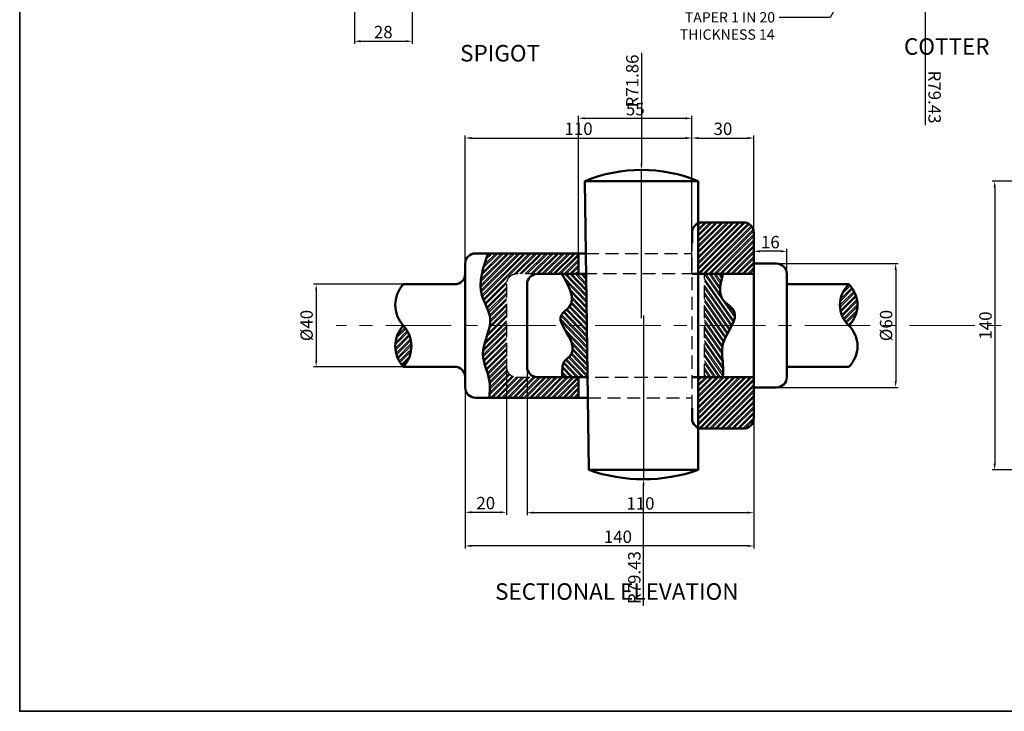
# Model space of a CAD drawing. Units: millimetres. Extents: x 641 to 1388, y -43 to 643.
# Tile 1 of 3: x 641 to 1119, y -43 to 293. Entities that reach past the tile are written whole.
import ezdxf
from ezdxf import colors
from ezdxf.entities.mleader import LeaderData, LeaderLine
from ezdxf.math import Vec2, Vec3

# ---------------------------------------------------------------- set-up
doc = ezdxf.new("R2010")
doc.units = ezdxf.units.MM
doc.linetypes.add('CENTER', pattern=[50.8, 31.75, -6.35, 6.35, -6.35])
doc.linetypes.add('HIDDEN', pattern=[9.525, 6.35, -3.175])
for name, color, linetype, lineweight in [('M-CNTR', 1, 'CENTER', 18), ('M-DIMS', 2, 'Continuous', 25), ('M-HATC', 8, 'Continuous', 18), ('M-HIDN', 4, 'HIDDEN', 25), ('M-OUTL', 7, 'Continuous', 50), ('M-TEXT', 3, 'Continuous', 25), ('M-TTLB', 7, 'Continuous', 35)]:
    doc.layers.add(name, color=color, linetype=linetype, lineweight=lineweight)
doc.styles.get("Standard").update_dxf_attribs({"font": 'arial.ttf'})
doc.dimstyles.new('ISO-25', dxfattribs={"dimtxt": 6, "dimasz": 3, "dimexe": 1.25, "dimexo": 0.625, "dimtad": 1, "dimdec": 0, "dimtxsty": 'Standard', "dimcen": 2.5, "dimadec": 0, "dimazin": 0, "dimtfac": 1, "dimtdec": 0, "dimtmove": 0, "dimatfit": 3, "dimfxl": 1, "dimarcsym": 0})
pattern_1 = [(45, (1327.4886, -130.5166), (-1.3470384, 1.3470384), []), (45, (1328.3867, -130.5166), (-1.3470384, 1.3470384), [])]

# ---------------------------------------------------------------- blocks, each defined once
blk = doc.blocks.new('*D18')
at = {"layer": 'Defpoints', "color": 0, "transparency": 16777216}
for p in [(836.38, 164.4), (785.11, 124.4), (836.38, 124.4)]:
    blk.add_point(p, dxfattribs=at)
at = {"layer": 'M-DIMS', "color": 0, "lineweight": -2, "transparency": 16777216}
for p, q in [((835.76, 164.4), (783.86, 164.4)), ((785.11, 161.4), (785.11, 127.4)), ((835.76, 124.4), (783.86, 124.4))]:
    blk.add_line(p, q, dxfattribs=at)
at = {"layer": 'M-DIMS', "color": 0, "transparency": 16777216}
for points in [[(784.61, 161.4), (785.61, 161.4), (785.11, 164.4)], [(784.61, 127.4), (785.61, 127.4), (785.11, 124.4)]]:
    blk.add_solid(points, dxfattribs=at)
at = {"layer": 'M-DIMS', "color": 0, "transparency": 16777216, "insert": (781.25, 144.4), "char_height": 6, "attachment_point": 5, "rotation": 90}
blk.add_mtext('%%C40', dxfattribs=at)
blk = doc.blocks.new('*D19')
at = {"layer": 'Defpoints', "color": 0, "transparency": 16777216}
for p in [(967.35, 235.32), (857.35, 169.4), (967.35, 169.4)]:
    blk.add_point(p, dxfattribs=at)
at = {"layer": 'M-DIMS', "color": 0, "lineweight": -2, "transparency": 16777216}
for p, q in [((857.35, 170.02), (857.35, 236.57)), ((860.35, 235.32), (964.35, 235.32)), ((967.35, 170.02), (967.35, 236.57))]:
    blk.add_line(p, q, dxfattribs=at)
at = {"layer": 'M-DIMS', "color": 0, "transparency": 16777216}
for points in [[(860.35, 235.82), (860.35, 234.82), (857.35, 235.32)], [(964.35, 235.82), (964.35, 234.82), (967.35, 235.32)]]:
    blk.add_solid(points, dxfattribs=at)
at = {"layer": 'M-DIMS', "color": 0, "transparency": 16777216, "insert": (912.35, 239.01), "char_height": 6, "attachment_point": 5}
blk.add_mtext('110', dxfattribs=at)
blk = doc.blocks.new('*D20')
at = {"layer": 'Defpoints', "color": 0, "transparency": 16777216}
for p in [(997.35, 235.31), (967.35, 221.9), (997.35, 181.87)]:
    blk.add_point(p, dxfattribs=at)
at = {"layer": 'M-DIMS', "color": 0, "lineweight": -2, "transparency": 16777216}
for p, q in [((967.35, 222.52), (967.35, 236.56)), ((970.35, 235.31), (994.35, 235.31)), ((997.35, 182.5), (997.35, 236.56))]:
    blk.add_line(p, q, dxfattribs=at)
at = {"layer": 'M-DIMS', "color": 0, "transparency": 16777216}
for points in [[(970.35, 235.81), (970.35, 234.81), (967.35, 235.31)], [(994.35, 235.81), (994.35, 234.81), (997.35, 235.31)]]:
    blk.add_solid(points, dxfattribs=at)
at = {"layer": 'M-DIMS', "color": 0, "transparency": 16777216, "insert": (982.35, 239), "char_height": 6, "attachment_point": 5}
blk.add_mtext('30', dxfattribs=at)
blk = doc.blocks.new('*D21')
at = {"layer": 'Defpoints', "color": 0, "transparency": 16777216}
for p in [(857.35, 129.03), (877.35, 129.03), (877.35, 53.85)]:
    blk.add_point(p, dxfattribs=at)
at = {"layer": 'M-DIMS', "color": 0, "lineweight": -2, "transparency": 16777216}
for p, q in [((857.35, 128.41), (857.35, 52.6)), ((877.35, 128.41), (877.35, 52.6)), ((860.35, 53.85), (874.35, 53.85))]:
    blk.add_line(p, q, dxfattribs=at)
at = {"layer": 'M-DIMS', "color": 0, "transparency": 16777216}
for points in [[(860.35, 54.35), (860.35, 53.35), (857.35, 53.85)], [(874.35, 54.35), (874.35, 53.35), (877.35, 53.85)]]:
    blk.add_solid(points, dxfattribs=at)
at = {"layer": 'M-DIMS', "color": 0, "transparency": 16777216, "insert": (867.35, 57.54), "char_height": 6, "attachment_point": 5}
blk.add_mtext('20', dxfattribs=at)
blk = doc.blocks.new('*D22')
at = {"layer": 'Defpoints', "color": 0, "transparency": 16777216}
for p in [(887.35, 133.67), (997.35, 133.67), (997.35, 53.67)]:
    blk.add_point(p, dxfattribs=at)
at = {"layer": 'M-DIMS', "color": 0, "lineweight": -2, "transparency": 16777216}
for p, q in [((887.35, 133.04), (887.35, 52.42)), ((997.35, 133.04), (997.35, 52.42)), ((890.35, 53.67), (994.35, 53.67))]:
    blk.add_line(p, q, dxfattribs=at)
at = {"layer": 'M-DIMS', "color": 0, "transparency": 16777216}
for points in [[(890.35, 54.17), (890.35, 53.17), (887.35, 53.67)], [(994.35, 54.17), (994.35, 53.17), (997.35, 53.67)]]:
    blk.add_solid(points, dxfattribs=at)
at = {"layer": 'M-DIMS', "color": 0, "transparency": 16777216, "insert": (942.35, 57.36), "char_height": 6, "attachment_point": 5}
blk.add_mtext('110', dxfattribs=at)
blk = doc.blocks.new('*D23')
at = {"layer": 'Defpoints', "color": 0, "transparency": 16777216}
for p in [(997.35, 133.67), (857.35, 61.79), (857.35, 37.53)]:
    blk.add_point(p, dxfattribs=at)
at = {"layer": 'M-DIMS', "color": 0, "lineweight": -2, "transparency": 16777216}
for p, q in [((997.35, 133.04), (997.35, 36.28)), ((857.35, 61.16), (857.35, 36.28)), ((994.35, 37.53), (860.35, 37.53))]:
    blk.add_line(p, q, dxfattribs=at)
at = {"layer": 'M-DIMS', "color": 0, "transparency": 16777216}
for points in [[(860.35, 38.03), (860.35, 37.03), (857.35, 37.53)], [(994.35, 38.03), (994.35, 37.03), (997.35, 37.53)]]:
    blk.add_solid(points, dxfattribs=at)
at = {"layer": 'M-DIMS', "color": 0, "transparency": 16777216, "insert": (931.43, 41.22), "char_height": 6, "attachment_point": 5}
blk.add_mtext('140', dxfattribs=at)
blk = doc.blocks.new('*D24')
at = {"layer": 'Defpoints', "color": 0, "transparency": 16777216}
for p in [(1002.85, 174.4), (1002.85, 114.4), (1066.11, 114.4)]:
    blk.add_point(p, dxfattribs=at)
at = {"layer": 'M-DIMS', "color": 0, "lineweight": -2, "transparency": 16777216}
for p, q in [((1003.48, 174.4), (1067.36, 174.4)), ((1066.11, 171.4), (1066.11, 117.4)), ((1003.48, 114.4), (1067.36, 114.4))]:
    blk.add_line(p, q, dxfattribs=at)
at = {"layer": 'M-DIMS', "color": 0, "transparency": 16777216}
for points in [[(1065.61, 171.4), (1066.61, 171.4), (1066.11, 174.4)], [(1065.61, 117.4), (1066.61, 117.4), (1066.11, 114.4)]]:
    blk.add_solid(points, dxfattribs=at)
at = {"layer": 'M-DIMS', "color": 0, "transparency": 16777216, "insert": (1062.25, 144.4), "char_height": 6, "attachment_point": 5, "rotation": 90}
blk.add_mtext('%%C60', dxfattribs=at)
blk = doc.blocks.new('*D25')
at = {"layer": 'Defpoints', "color": 0, "transparency": 16777216}
for p in [(997.35, 180.38), (997.35, 164.4), (1013.35, 164.4)]:
    blk.add_point(p, dxfattribs=at)
at = {"layer": 'M-DIMS', "color": 0, "lineweight": -2, "transparency": 16777216}
for p, q in [((997.35, 165.02), (997.35, 181.63)), ((1013.35, 165.02), (1013.35, 181.63)), ((1010.35, 180.38), (1000.35, 180.38))]:
    blk.add_line(p, q, dxfattribs=at)
at = {"layer": 'M-DIMS', "color": 0, "transparency": 16777216}
for points in [[(1000.35, 180.88), (1000.35, 179.88), (997.35, 180.38)], [(1010.35, 180.88), (1010.35, 179.88), (1013.35, 180.38)]]:
    blk.add_solid(points, dxfattribs=at)
at = {"layer": 'M-DIMS', "color": 0, "transparency": 16777216, "insert": (1005.35, 184.07), "char_height": 6, "attachment_point": 5}
blk.add_mtext('16', dxfattribs=at)
blk = doc.blocks.new('*D26')
at = {"layer": 'Defpoints', "color": 0, "transparency": 16777216}
for p in [(1174.83, 214.4), (1114.12, 74.4), (1174.83, 74.4)]:
    blk.add_point(p, dxfattribs=at)
at = {"layer": 'M-DIMS', "color": 0, "lineweight": -2, "transparency": 16777216}
for p, q in [((1174.21, 214.4), (1112.87, 214.4)), ((1114.12, 211.4), (1114.12, 77.4)), ((1174.21, 74.4), (1112.87, 74.4))]:
    blk.add_line(p, q, dxfattribs=at)
at = {"layer": 'M-DIMS', "color": 0, "transparency": 16777216}
for points in [[(1113.62, 211.4), (1114.62, 211.4), (1114.12, 214.4)], [(1113.62, 77.4), (1114.62, 77.4), (1114.12, 74.4)]]:
    blk.add_solid(points, dxfattribs=at)
at = {"layer": 'M-DIMS', "color": 0, "transparency": 16777216, "insert": (1110.43, 144.4), "char_height": 6, "attachment_point": 5, "rotation": 90}
blk.add_mtext('140', dxfattribs=at)
blk = doc.blocks.new('COTTER')
for p, q in [((0, 144.55), (55, 144.55)), ((2, 4.55), (0, 144.55)), ((55, 144.55), (55, 4.55)), ((55, 4.55), (2, 4.55)), ((2, 4.55), (4, 4.55)), ((2, 4.55), (4, 4.55))]:
    blk.add_line(p, q)
for centre, radius, start, end in [((27.5, 78.16), 71.86, 67.5, 112.5), ((28.5, 79.43), 79.43, 250.5117, 289.4883)]:
    blk.add_arc(centre, radius, start, end)
blk = doc.blocks.new('*D31')
at = {"layer": 'Defpoints', "color": 0, "transparency": 16777216}
for p in [(967.35, 244.87), (912.35, 179.4), (967.35, 179.4)]:
    blk.add_point(p, dxfattribs=at)
at = {"layer": 'M-DIMS', "color": 0, "lineweight": -2, "transparency": 16777216}
for p, q in [((912.35, 180.02), (912.35, 246.12)), ((915.35, 244.87), (964.35, 244.87)), ((967.35, 180.02), (967.35, 246.12))]:
    blk.add_line(p, q, dxfattribs=at)
at = {"layer": 'M-DIMS', "color": 0, "transparency": 16777216}
for points in [[(915.35, 245.37), (915.35, 244.37), (912.35, 244.87)], [(964.35, 245.37), (964.35, 244.37), (967.35, 244.87)]]:
    blk.add_solid(points, dxfattribs=at)
at = {"layer": 'M-DIMS', "color": 0, "transparency": 16777216, "insert": (939.85, 248.54), "char_height": 6, "attachment_point": 5}
blk.add_mtext('55', dxfattribs=at)
blk = doc.blocks.new('*D32')
at = {"layer": 'Defpoints', "color": 0, "transparency": 16777216}
for p in [(803.65, 333.79), (831.65, 328.79), (831.65, 282.23)]:
    blk.add_point(p, dxfattribs=at)
at = {"layer": 'M-DIMS', "color": 0, "lineweight": -2, "transparency": 16777216}
for p, q in [((803.65, 333.16), (803.65, 280.98)), ((831.65, 328.16), (831.65, 280.98)), ((806.65, 282.23), (828.65, 282.23))]:
    blk.add_line(p, q, dxfattribs=at)
at = {"layer": 'M-DIMS', "color": 0, "transparency": 16777216}
for points in [[(806.65, 282.73), (806.65, 281.73), (803.65, 282.23)], [(828.65, 282.73), (828.65, 281.73), (831.65, 282.23)]]:
    blk.add_solid(points, dxfattribs=at)
at = {"layer": 'M-DIMS', "color": 0, "transparency": 16777216, "insert": (817.65, 285.91), "char_height": 6, "attachment_point": 5}
blk.add_mtext('28', dxfattribs=at)
blk = doc.blocks.new('*D33')
at = {"layer": 'Defpoints', "color": 0, "transparency": 16777216}
for p in [(1080.53, 382.26), (1080.53, 302.83)]:
    blk.add_point(p, dxfattribs=at)
at = {"layer": 'M-DIMS', "color": 0, "lineweight": -2, "transparency": 16777216}
for p, q in [((1080.53, 382.26), (1080.53, 302.83)), ((1080.53, 241.55), (1080.53, 299.83))]:
    blk.add_line(p, q, dxfattribs=at)
at = {"layer": 'M-DIMS', "color": 0, "transparency": 16777216}
blk.add_solid([(1081.03, 299.83), (1080.03, 299.83), (1080.53, 302.83)], dxfattribs=at)
at = {"layer": 'M-DIMS', "color": 0, "transparency": 16777216, "insert": (1084.22, 255.17), "char_height": 6, "attachment_point": 5, "rotation": 270.0002}
blk.add_mtext('R79.43', dxfattribs=at)
blk = doc.blocks.new('*D35')
at = {"layer": 'Defpoints', "color": 0, "transparency": 16777216}
for p in [(943.85, 149.28), (943.85, 69.85)]:
    blk.add_point(p, dxfattribs=at)
at = {"layer": 'M-DIMS', "color": 0, "lineweight": -2, "transparency": 16777216}
for p, q in [((943.85, 149.28), (943.85, 69.85)), ((943.85, 8.57), (943.85, 66.85))]:
    blk.add_line(p, q, dxfattribs=at)
at = {"layer": 'M-DIMS', "color": 0, "transparency": 16777216}
blk.add_solid([(943.36, 66.85), (944.36, 66.85), (943.85, 69.85)], dxfattribs=at)
at = {"layer": 'M-DIMS', "color": 0, "transparency": 16777216, "insert": (940.16, 22.19), "char_height": 6, "attachment_point": 5, "rotation": 90}
blk.add_mtext('R79.43', dxfattribs=at)
blk = doc.blocks.new('*D36')
at = {"layer": 'Defpoints', "color": 0, "transparency": 16777216}
for p in [(942.85, 219.87), (942.85, 148.01)]:
    blk.add_point(p, dxfattribs=at)
at = {"layer": 'M-DIMS', "color": 0, "lineweight": -2, "transparency": 16777216}
for p, q in [((942.85, 276.6), (942.85, 222.87)), ((942.85, 148.01), (942.85, 219.87))]:
    blk.add_line(p, q, dxfattribs=at)
at = {"layer": 'M-DIMS', "color": 0, "transparency": 16777216}
blk.add_solid([(942.36, 222.87), (943.36, 222.87), (942.85, 219.87)], dxfattribs=at)
at = {"layer": 'M-DIMS', "color": 0, "transparency": 16777216, "insert": (939.17, 262.98), "char_height": 6, "attachment_point": 5, "rotation": 90}
blk.add_mtext('R71.86', dxfattribs=at)

msp = doc.modelspace()

# ---------------------------------------------------------------- hatches: boundary and pattern name
at = {"layer": 'M-HATC'}
h = msp.add_hatch(dxfattribs=at)
h.set_pattern_fill('ANSI32', color=256, scale=0.2)
h.set_pattern_definition(pattern_1)
h.paths.add_polyline_path([(970.355, 119.396), (970.355, 94.813, 0.1032437), (972.355, 94.396), (992.355, 94.396, 0.4142136), (997.355, 99.396), (997.355, 119.396)])
h.paths.add_polyline_path([(970.355, 193.979), (970.355, 169.396), (997.355, 169.396), (997.355, 174.396), (997.355, 189.396, 0.4142136), (992.355, 194.396), (972.355, 194.396, 0.1032437)])
h = msp.add_hatch(dxfattribs=at)
h.set_pattern_fill('ANSI32', color=256, scale=0.2)
h.set_pattern_definition(pattern_1)
edge = h.paths.add_edge_path()
edge.add_line((882.355, 169.396), (912.355, 169.396))
edge.add_line((912.355, 169.396), (912.355, 179.396))
edge.add_line((912.355, 179.396), (868.372, 179.396))
edge.add_spline(control_points=[(868.372, 179.396), (866.017, 172.5), (862.281, 161.563), (869.872, 150.51), (869.52, 145.522), (869.328, 144.396)], knot_values=[0, 0, 0, 0, 20.5117466, 32.5267505, 35.9980813, 35.9980813, 35.9980813, 35.9980813], degree=3, periodic=0)
edge.add_line((869.328, 144.396), (877.355, 144.396))
edge.add_line((877.355, 144.396), (877.355, 164.396))
edge.add_arc((882.355, 164.396), 5, 90, 180, ccw=False)
edge = h.paths.add_edge_path()
edge.add_line((877.355, 144.396), (869.328, 144.396))
edge.add_spline(control_points=[(869.328, 144.396), (868.545, 139.814), (863.452, 130.794), (869.899, 119.498), (869.301, 112.279), (869.063, 109.396)], knot_values=[35.9980813, 35.9980813, 35.9980813, 35.9980813, 50.1240233, 63.0337908, 71.6192278, 71.6192278, 71.6192278, 71.6192278], degree=3, periodic=0)
edge.add_line((869.063, 109.396), (912.355, 109.396))
edge.add_line((912.355, 109.396), (912.355, 119.396))
edge.add_line((912.355, 119.396), (892.355, 119.396))
edge.add_line((892.355, 119.396), (882.355, 119.396))
edge.add_arc((882.355, 124.396), 5, 180, 270, ccw=False)
edge.add_line((877.355, 124.396), (877.355, 144.396))
h = msp.add_hatch(dxfattribs=at)
h.set_pattern_fill('ANSI32', color=256, scale=0.2, angle=89)
h.set_pattern_definition([(134, (1327.4886, -130.5166), (-1.370342, -1.323324), []), (134, (1327.5043, -129.6187), (-1.370342, -1.323324), [])])
edge = h.paths.add_edge_path()
edge.add_line((915.998, 169.396), (904.176, 169.396))
edge.add_spline(control_points=[(904.176, 169.396), (907.692, 163.365), (912.308, 155.445), (902.688, 149.532), (903.614, 146.308), (904.603, 144.396)], knot_values=[0, 0, 0, 0, 16.5553178, 21.7400198, 27.8381389, 27.8381389, 27.8381389, 27.8381389], degree=3, periodic=0)
edge.add_line((904.603, 144.396), (916.355, 144.396))
edge.add_line((916.355, 144.396), (915.998, 169.396))
edge = h.paths.add_edge_path()
edge.add_line((916.355, 144.396), (904.603, 144.396))
edge.add_spline(control_points=[(904.603, 144.396), (905.728, 142.22), (909.307, 137.342), (910.04, 130.547), (904.064, 126.789), (904.343, 122.39), (904.534, 119.396)], knot_values=[27.8381389, 27.8381389, 27.8381389, 27.8381389, 34.7758747, 41.9663082, 45.7817706, 53.9156246, 53.9156246, 53.9156246, 53.9156246], degree=3, periodic=0)
edge.add_line((904.534, 119.396), (916.712, 119.396))
edge.add_line((916.712, 119.396), (916.355, 144.396))
h = msp.add_hatch(dxfattribs=at)
h.set_pattern_fill('ANSI32', color=256, scale=0.2, angle=80)
h.set_pattern_definition([(125, (1327.4886, -130.5166), (-1.560485, -1.092663), []), (125, (1327.6446, -129.6322), (-1.560485, -1.092663), [])])
edge = h.paths.add_edge_path()
edge.add_spline(control_points=[(986.628, 144.396), (987.993, 147.081), (989.617, 151.846), (979.205, 157.416), (981.144, 164.79), (982.355, 169.396)], knot_values=[0, 0, 0, 0, 8.2277099, 15.729056, 28.2082665, 28.2082665, 28.2082665, 28.2082665], degree=3, periodic=0)
edge.add_line((982.355, 169.396), (973.355, 169.396))
edge.add_line((973.355, 169.396), (973.355, 144.396))
edge.add_line((973.355, 144.396), (986.628, 144.396))
edge = h.paths.add_edge_path()
edge.add_spline(control_points=[(982.355, 119.396), (982.416, 121.513), (982.571, 126.882), (980.866, 135.03), (985.173, 141.532), (986.628, 144.396)], knot_values=[28.2082665, 28.2082665, 28.2082665, 28.2082665, 34.5448861, 44.2761211, 53.0497567, 53.0497567, 53.0497567, 53.0497567], degree=3, periodic=0)
edge.add_line((986.628, 144.396), (973.355, 144.396))
edge.add_line((973.355, 144.396), (973.355, 119.396))
edge.add_line((973.355, 119.396), (982.355, 119.396))
h = msp.add_hatch(dxfattribs=at)
h.set_pattern_fill('ANSI32', color=256, scale=0.2)
h.set_pattern_definition([(45, (803.6772, 471.05), (-1.347038, 1.347038), []), (45, (804.5752, 471.05), (-1.347038, 1.347038), [])])
h.paths.add_polyline_path([(1043.355, 144.396, 0.4249028), (1043.355, 164.396, 0.4249028)])
h = msp.add_hatch(dxfattribs=at)
h.set_pattern_fill('ANSI32', color=256, scale=0.2)
h.set_pattern_definition(pattern_1)
h.paths.add_polyline_path([(827.355, 124.396, 0.3912814), (827.355, 144.396, 0.3912814)])

# ---------------------------------------------------------------- linework, layer by layer
at = {"layer": 'M-CNTR'}
msp.add_line((1256.973, 144.396), (794.875, 144.396), dxfattribs=at)
at = {"layer": 'M-HIDN'}
for p, q in [((967.355, 104.396), (967.355, 184.396)), ((915.855, 179.396), (967.355, 179.396)), ((973.355, 119.396), (973.355, 169.396)), ((916.855, 109.396), (967.355, 109.396))]:
    msp.add_line(p, q, dxfattribs=at)
msp.add_lwpolyline([(997.355, 169.396), (882.355, 169.396, 0.4142136), (877.355, 164.396), (877.355, 124.396, 0.4142136), (882.355, 119.396), (997.355, 119.396)], format="xyb", dxfattribs=at)
at = {"layer": 'M-OUTL'}
for p, q in [((970.355, 94.813), (970.355, 193.979)), ((972.355, 194.396), (992.355, 194.396)), ((967.355, 184.396), (967.355, 189.396)), ((997.355, 189.396), (997.355, 99.396)), ((862.355, 179.396), (915.855, 179.396)), ((912.355, 169.396), (912.355, 179.396)), ((857.355, 169.396), (857.355, 174.396)), ((1008.355, 174.396), (997.355, 174.396)), ((997.355, 174.396), (997.355, 114.396)), ((857.355, 114.396), (857.355, 169.396)), ((892.355, 169.396), (915.998, 169.396)), ((967.355, 169.396), (997.355, 169.396)), ((1013.355, 119.396), (1013.355, 169.396)), ((852.355, 164.396), (827.355, 164.396)), ((887.355, 124.396), (887.355, 164.396)), ((1013.355, 164.396), (1043.355, 164.396)), ((827.355, 124.396), (852.355, 124.396)), ((1043.355, 124.396), (1013.355, 124.396)), ((892.355, 119.396), (916.712, 119.396)), ((912.355, 109.396), (912.355, 119.396)), ((967.355, 119.396), (997.355, 119.396)), ((997.355, 114.396), (1008.355, 114.396)), ((862.355, 109.396), (916.855, 109.396)), ((967.355, 99.396), (967.355, 104.396)), ((992.355, 94.396), (972.355, 94.396))]:
    msp.add_line(p, q, dxfattribs=at)
for centre, radius, start, end in [((972.355, 189.396), 5, 90, 180), ((992.355, 189.396), 5, 0, 90), ((862.355, 174.396), 5, 90, 180), ((1008.355, 169.396), 5, 0, 90), ((852.355, 169.396), 5, 270, 0), ((892.355, 164.396), 5, 90, 180), ((838.177, 154.396), 14.735, 137.26103, 222.73897), ((1052.998, 154.396), 13.892, 133.95845, 226.04155), ((1033.712, 154.396), 13.892, 313.95845, 46.04155), ((838.177, 134.396), 14.735, 137.26103, 222.73897), ((816.533, 134.396), 14.735, 317.26103, 42.73897), ((1033.712, 134.396), 13.892, 313.95845, 46.04155), ((852.355, 119.396), 5, 0, 90), ((892.355, 124.396), 5, 180, 270), ((1008.355, 119.396), 5, 270, 0), ((862.355, 114.396), 5, 180, 270), ((972.355, 99.396), 5, 180, 270), ((992.355, 99.396), 5, 270, 0)]:
    msp.add_arc(centre, radius, start, end, dxfattribs=at)
for points, knots in [([(868.372, 179.396), (866.017, 172.5), (862.281, 161.563), (872.851, 146.172), (862.824, 131.895), (869.899, 119.498), (869.301, 112.279), (869.063, 109.396)], [0, 0, 0, 0, 20.5117466, 32.5267505, 50.1240233, 63.0337908, 71.6192278, 71.6192278, 71.6192278, 71.6192278]), ([(904.176, 169.396), (907.692, 163.365), (912.308, 155.445), (900.291, 148.059), (909.058, 139.652), (910.04, 130.547), (904.064, 126.789), (904.343, 122.39), (904.534, 119.396)], [0, 0, 0, 0, 16.5553178, 21.7400198, 34.7758747, 41.9663082, 45.7817706, 53.9156246, 53.9156246, 53.9156246, 53.9156246]), ([(982.355, 169.396), (981.144, 164.79), (979.205, 157.416), (992.856, 150.114), (980.302, 137.729), (982.571, 126.882), (982.416, 121.513), (982.355, 119.396)], [0, 0, 0, 0, 12.4792105, 19.9805566, 36.981902, 46.713137, 53.0497567, 53.0497567, 53.0497567, 53.0497567])]:
    msp.add_open_spline(points, degree=3, knots=knots, dxfattribs=at)
at = {"layer": 'M-TTLB'}
msp.add_lwpolyline([(641.348, 642.837), (1388.388, 642.837), (1388.388, -42.647), (641.348, -42.647)], close=True, dxfattribs=at)

# ---------------------------------------------------------------- block references
at = {"layer": 'M-OUTL'}
msp.add_blockref('COTTER', (915.355, 69.846), dxfattribs=at)

# ---------------------------------------------------------------- texts
at = {"layer": 'M-TEXT', "char_height": 8, "attachment_point": 1}
for s, width, insert in [('\\pxqc;COTTER', 68.77128, (1056.492, 283.704)), ('\\pxqc;SPIGOT', 125.14088, (811.709, 280.436)), ('\\pxqc;SECTIONAL ELEVATION', 131.26047, (865.253, 19.433))]:
    msp.add_mtext_dynamic_manual_height_columns(s, width=width, gutter_width=12.5, heights=[0], dxfattribs=dict(at, insert=insert))

# ---------------------------------------------------------------- dimensions: what is measured, and where the dimension line sits
at = {"layer": 'M-DIMS'}
for center, mpoint, picture, middle in [((1080.53, 382.259), (1080.53, 302.826), '*D33', (1080.53, 255.166)), ((942.855, 148.005), (942.855, 219.866), '*D36', (942.855, 262.983)), ((943.855, 149.278), (943.855, 69.845), '*D35', (943.855, 22.185))]:
    dim = msp.add_radius_dim(center=center, mpoint=mpoint, dimstyle='ISO-25', override={"dimdec": 2, "dimlfac": 1, "dimrnd": 0, "dimzin": 0, "dimdsep": 46, "dimlunit": 2}, dxfattribs=at)
    dim.commit()
    dim.dimension.update_dxf_attribs({"geometry": picture, "text_midpoint": middle, "dimtype": 164})
for base, p1, p2, override, picture, middle in [((831.65, 282.226), (803.65, 333.786), (831.65, 328.786), {"dimdec": 0, "dimlfac": 1, "dimrnd": 0, "dimzin": 0, "dimdsep": 46, "dimlunit": 2}, '*D32', (817.65, 285.914)), ((967.355, 244.866), (912.355, 179.396), (967.355, 179.396), {"dimdec": 0, "dimlfac": 1, "dimrnd": 0, "dimzin": 0, "dimdsep": 46, "dimlunit": 2}, '*D31', (939.855, 248.542)), ((967.355, 235.324), (857.355, 169.396), (967.355, 169.396), {"dimclrd": 0, "dimclre": 0, "dimclrt": 0}, '*D19', (912.355, 239.013)), ((997.355, 235.314), (967.355, 221.898), (997.355, 181.875), {"dimclrd": 0, "dimclre": 0, "dimclrt": 0}, '*D20', (982.355, 239.005)), ((997.355, 180.379), (1013.355, 164.396), (997.355, 164.396), {"dimclrd": 0, "dimclre": 0, "dimclrt": 0}, '*D25', (1005.355, 184.068))]:
    dim = msp.add_linear_dim(base=base, p1=p1, p2=p2, dimstyle='ISO-25', override=override, dxfattribs=at)
    dim.commit()
    dim.dimension.update_dxf_attribs({"geometry": picture, "text_midpoint": middle})
dim = msp.add_linear_dim(base=(1114.115, 74.396), p1=(1174.832, 214.396), p2=(1174.832, 74.396), angle=90, dimstyle='ISO-25', override={"dimclrd": 0, "dimclre": 0, "dimclrt": 0}, dxfattribs=at)
dim.commit()
dim.dimension.update_dxf_attribs({"geometry": '*D26', "text_midpoint": (1110.427, 144.396)})
for base, p1, p2, picture, middle in [((1066.108, 114.396), (1002.855, 174.396), (1002.855, 114.396), '*D24', (1062.252, 144.396)), ((785.108, 124.396), (836.381, 164.396), (836.381, 124.396), '*D18', (781.252, 144.396))]:
    dim = msp.add_linear_dim(base=base, p1=p1, p2=p2, angle=90, text='%%C<>', dimstyle='ISO-25', override={"dimclrd": 0, "dimclre": 0, "dimclrt": 0}, dxfattribs=at)
    dim.commit()
    dim.dimension.update_dxf_attribs({"geometry": picture, "text_midpoint": middle})
for base, p1, p2, picture, middle in [((857.355, 37.528), (997.355, 133.669), (857.355, 61.787), '*D23', (931.431, 37.528)), ((877.355, 53.852), (857.355, 129.033), (877.355, 129.033), '*D21', (867.355, 53.852)), ((997.355, 53.67), (887.355, 133.669), (997.355, 133.669), '*D22', (942.355, 53.67))]:
    dim = msp.add_linear_dim(base=base, p1=p1, p2=p2, dimstyle='ISO-25', override={"dimclrd": 0, "dimclre": 0, "dimclrt": 0}, dxfattribs=at)
    dim.commit()
    dim.dimension.update_dxf_attribs({"geometry": picture, "text_midpoint": middle, "dimtype": 160})

# ---------------------------------------------------------------- leaders
at = {"layer": 'M-TEXT'}
ml = msp.add_multileader_mtext('Standard', dxfattribs=at)
ml.set_content('TAPER 1 IN 20 \\P\\pxqc;THICKNESS 14', color=256)
ml.set_leader_properties()
ml.build(insert=Vec2(0, 0))
ctx = ml.context
ctx.base_point, ctx.char_height, ctx.plane_origin = Vec3(956.457, 293.786), 5, Vec3(1053.733, 328.138)
ctx.text_align_type = 2
notes = []
notes.append((ctx, [(0, (1, 1, 0), (1034.33, 293.786), (-1, 0), 24.688, [(0, [(1053.733, 328.138)], 0, [])])]))
ctx.mtext.insert, ctx.mtext.alignment, ctx.mtext.flow_direction = Vec3(1007.642, 296.329), 3, 5
for ctx, leaders in notes:
    for number, flags, end, landing, length, lines in leaders:
        leader = LeaderData()
        leader.index, (leader.has_last_leader_line, leader.has_dogleg_vector, leader.attachment_direction) = number, flags
        leader.last_leader_point, leader.dogleg_vector, leader.dogleg_length = Vec3(end), Vec3(landing), length
        for number, points, colour, breaks in lines:
            line = LeaderLine()
            line.index, line.vertices, line.color, line.breaks = number, Vec3.list(points), colors.encode_raw_color(colour), breaks
            leader.lines.append(line)
        ctx.leaders.append(leader)

doc.saveas('drawing.dxf')
